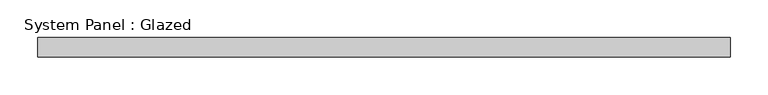
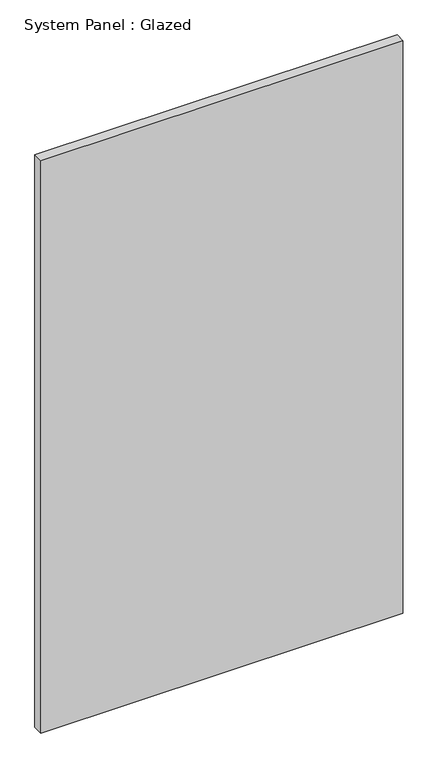
"""IFC4 building model written with IfcOpenShell, lengths in millimetres: plate geometry, System Panel : Glazed."""

from ifc_helpers import new_model, si_unit, origin, origin_with_axes, place, context, project, spatial, polyline, outline, extrude, source, transform, mapped, element, save


def system_panel_glazed_aa593011(model_context):
    return source(origin(), model_context, "Body", "SweptSolid", [
        extrude(outline(polyline([(455.6125, 19.05), (-455.6125, 19.05), (-455.6125, 44.45), (455.6125, 44.45), (455.6125, 19.05)])), origin_with_axes(), (0.0, 0.0, 1.0), 1522.5904225),
    ])


if __name__ == "__main__":
    model = new_model("IFC4")
    model_context = context("Model", 3, world=origin())
    ifc_project = project(units=[si_unit("LENGTHUNIT", "METRE", prefix="MILLI")], contexts=[model_context])
    site = spatial("IfcSite", under=ifc_project)
    building = spatial("IfcBuilding", under=site)
    placement = place(None, origin())
    system_panel_glazed_shape = system_panel_glazed_aa593011(model_context)
    element("IfcPlate", 1, ObjectType="System Panel : Glazed", at=placement, inside=building, context=model_context, shape_type="MappedRepresentation", body=[
        mapped(system_panel_glazed_shape, transform((0.0, 0.0, 0.0), x_axis=(1.0, 0.0, 0.0), y_axis=(0.0, 1.0, 0.0), z_axis=(0.0, 0.0, 1.0))),
    ])
    save(model, "model.ifc")

# Revit data of these elements
# Type "System Panel : Glazed"
#   Construction Type Id = "GSP4R"
#   Analytic Construction = "1/8 in Pilkington single glazing"
#   Visual Light Transmittance = 0.9
#   Solar Heat Gain Coefficient = 0.86
#   Heat Transfer Coefficient (U) = 1.18115 BTU/(h·ft²·°F)
#   Define Thermal Properties by = 1
# Element 1 (IfcPlate, "System Panel : Glazed")
#   Materials on its faces: "Glass"
# Materials
#   "Glass": class "Glass", colour RGB 0 128 192, transparency 0.75, Description = "Soda Lime Glass", Cost = 0
